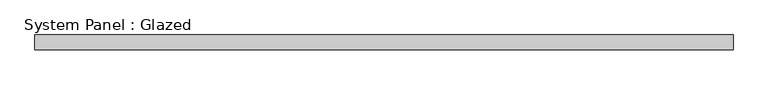
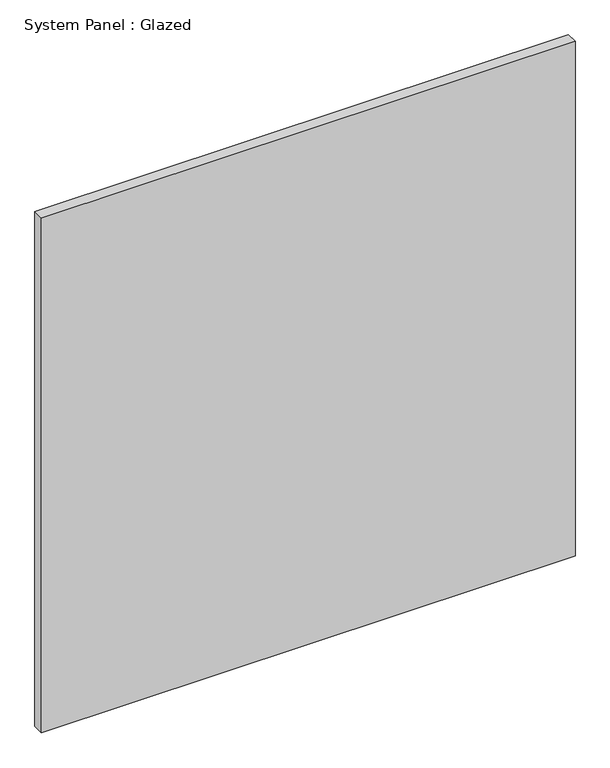
"""IFC4 building model written with IfcOpenShell, lengths in millimetres: plate geometry, System Panel : Glazed."""

from ifc_helpers import new_model, si_unit, origin, origin_with_axes, place, context, project, spatial, polyline, outline, extrude, source, transform, mapped, element, save


def system_panel_glazed_8157f083(model_context):
    return source(origin(), model_context, "Body", "SweptSolid", [
        extrude(outline(polyline([(597.3764963, 19.05), (-597.3764963, 19.05), (-597.3764963, 44.45), (597.3764963, 44.45), (597.3764963, 19.05)])), origin_with_axes(), (0.0, 0.0, 1.0), 1219.2),
    ])


if __name__ == "__main__":
    model = new_model("IFC4")
    model_context = context("Model", 3, world=origin())
    ifc_project = project(units=[si_unit("LENGTHUNIT", "METRE", prefix="MILLI")], contexts=[model_context])
    site = spatial("IfcSite", under=ifc_project)
    building = spatial("IfcBuilding", under=site)
    placement = place(None, origin())
    system_panel_glazed_shape = system_panel_glazed_8157f083(model_context)
    element("IfcPlate", 1, ObjectType="System Panel : Glazed", at=placement, inside=building, context=model_context, shape_type="MappedRepresentation", body=[
        mapped(system_panel_glazed_shape, transform((0.0, 0.0, 0.0), x_axis=(1.0, 0.0, 0.0), y_axis=(0.0, 1.0, 0.0), z_axis=(0.0, 0.0, 1.0))),
    ])
    save(model, "model.ifc")

# Revit data of these elements
# Type "System Panel : Glazed"
#   Construction Type Id = "GSP4R"
#   Analytic Construction = "1/8 in Pilkington single glazing"
#   Visual Light Transmittance = 0.9
#   Solar Heat Gain Coefficient = 0.86
#   Heat Transfer Coefficient (U) = 1.18115 BTU/(h·ft²·°F)
# Element 1 (IfcPlate, "System Panel : Glazed")
#   Materials on its faces: "Glass"
# Materials
#   "Glass": class "Glass", colour RGB 0 128 192, transparency 0.75, Description = "Soda Lime Glass", Cost = 0
